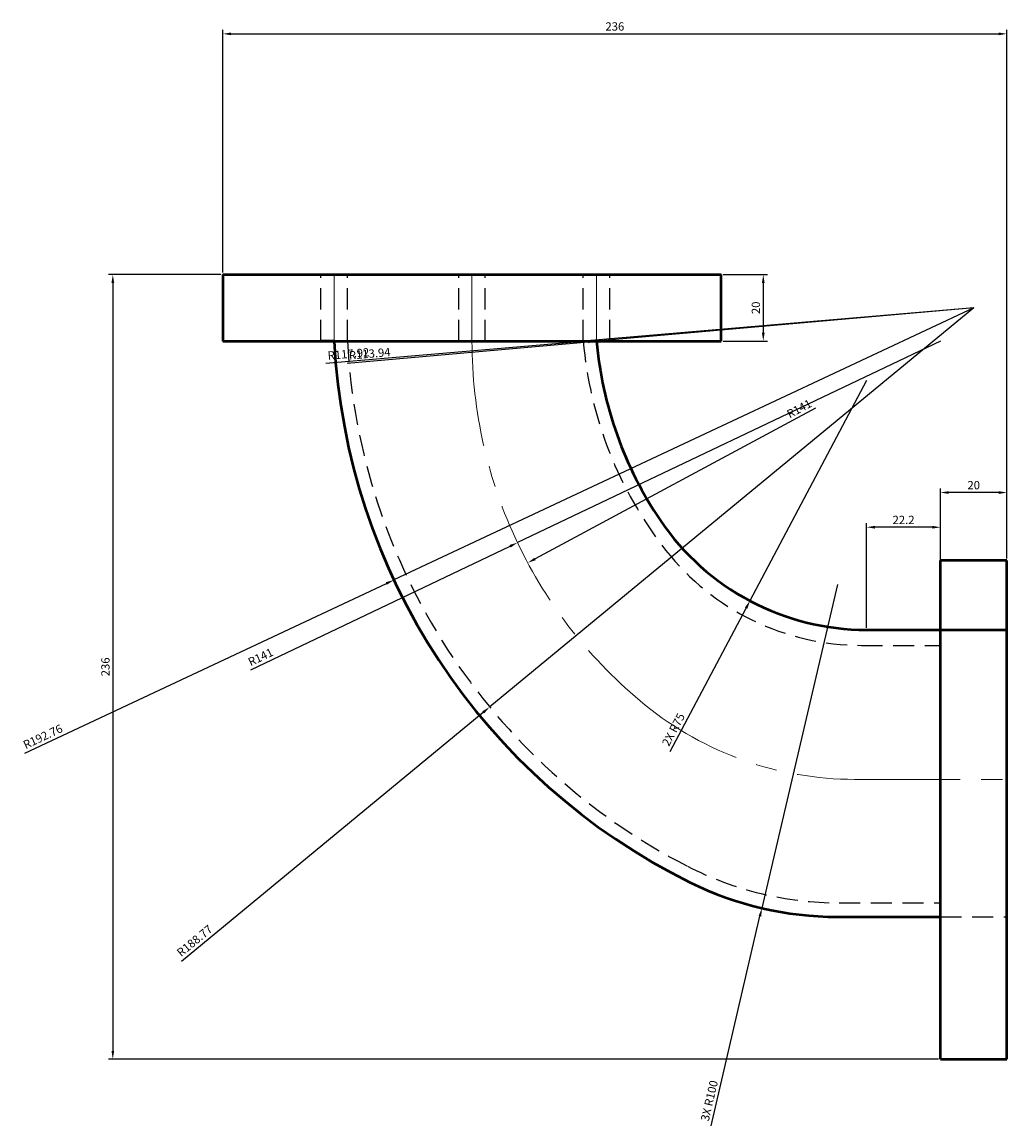
# Model space of a CAD drawing. Units: millimetres. Extents: x 1880 to 2565, y 1372 to 1704.
# Tile 1 of 2: x 1880 to 2176, y 1372 to 1704. Entities that reach past the tile are written whole.
import ezdxf

# ---------------------------------------------------------------- set-up
doc = ezdxf.new("R2010")
doc.units = ezdxf.units.MM
doc.linetypes.add('CENTER', pattern=[50.8, 31.75, -6.35, 6.35, -6.35])
doc.linetypes.add('HIDDEN', pattern=[9.525, 6.35, -3.175])
for name, color, linetype, lineweight in [('M-CNTR', 4, 'CENTER', 18), ('M-DIMS', 2, 'Continuous', 25), ('M-HIDN', 8, 'HIDDEN', 25), ('M-OUTL', 7, 'Continuous', 50)]:
    doc.layers.add(name, color=color, linetype=linetype, lineweight=lineweight)
doc.styles.get("Standard").update_dxf_attribs({"font": 'arial.ttf'})
doc.dimstyles.new('ISO-25', dxfattribs={"dimtxt": 2.5, "dimasz": 2.5, "dimexe": 1.25, "dimexo": 0.625, "dimtad": 1, "dimdec": 1, "dimdsep": 46, "dimtxsty": 'Standard', "dimcen": 2.5, "dimadec": 0, "dimazin": 0, "dimtfac": 1, "dimtdec": 1, "dimtmove": 0, "dimatfit": 3, "dimfxl": 1, "dimarcsym": 0})

# ---------------------------------------------------------------- blocks, each defined once
blk = doc.blocks.new('*D9')
at = {"layer": 'Defpoints', "color": 0, "lineweight": 100, "transparency": 16777216}
for p in [(2155.98, 1607.95), (2031.76, 1541.23)]:
    blk.add_point(p, dxfattribs=at)
at = {"layer": 'M-DIMS', "color": 0, "lineweight": -2, "transparency": 16777216}
blk.add_line((2118.32, 1587.72), (2033.97, 1542.42), dxfattribs=at)
at = {"layer": 'M-DIMS', "color": 0, "lineweight": 100, "transparency": 16777216}
blk.add_solid([(2033.77, 1542.78), (2034.16, 1542.05), (2031.76, 1541.23)], dxfattribs=at)
at = {"layer": 'M-DIMS', "color": 0, "transparency": 16777216, "insert": (2113.61, 1587.32), "char_height": 2.5, "attachment_point": 5, "rotation": 28.2384}
blk.add_mtext('R141', dxfattribs=at)
blk = doc.blocks.new('*D10')
at = {"layer": 'Defpoints', "color": 0, "lineweight": 100, "transparency": 16777216}
for p in [(2089.98, 1627.95), (2089.98, 1607.95), (2102.65, 1607.95)]:
    blk.add_point(p, dxfattribs=at)
at = {"layer": 'M-DIMS', "color": 0, "lineweight": -2, "transparency": 16777216}
for p, q in [((2090.61, 1627.95), (2103.9, 1627.95)), ((2102.65, 1625.45), (2102.65, 1610.45)), ((2090.61, 1607.95), (2103.9, 1607.95))]:
    blk.add_line(p, q, dxfattribs=at)
at = {"layer": 'M-DIMS', "color": 0, "lineweight": 100, "transparency": 16777216}
for points in [[(2102.23, 1625.45), (2103.06, 1625.45), (2102.65, 1627.95)], [(2102.23, 1610.45), (2103.06, 1610.45), (2102.65, 1607.95)]]:
    blk.add_solid(points, dxfattribs=at)
at = {"layer": 'M-DIMS', "color": 0, "transparency": 16777216, "insert": (2100.74, 1617.95), "char_height": 2.5, "attachment_point": 5, "rotation": 90}
blk.add_mtext('20', dxfattribs=at)
blk = doc.blocks.new('*D11')
at = {"layer": 'Defpoints', "color": 0, "lineweight": 100, "transparency": 16777216}
for p in [(2133.76, 1551.95), (2133.76, 1521.08), (2155.98, 1521.08)]:
    blk.add_point(p, dxfattribs=at)
at = {"layer": 'M-DIMS', "color": 0, "lineweight": -2, "transparency": 16777216}
for p, q in [((2133.76, 1521.71), (2133.76, 1553.2)), ((2153.48, 1551.95), (2136.26, 1551.95)), ((2155.98, 1521.71), (2155.98, 1553.2))]:
    blk.add_line(p, q, dxfattribs=at)
at = {"layer": 'M-DIMS', "color": 0, "lineweight": 100, "transparency": 16777216}
for points in [[(2136.26, 1552.36), (2136.26, 1551.53), (2133.76, 1551.95)], [(2153.48, 1552.36), (2153.48, 1551.53), (2155.98, 1551.95)]]:
    blk.add_solid(points, dxfattribs=at)
at = {"layer": 'M-DIMS', "color": 0, "transparency": 16777216, "insert": (2144.87, 1553.83), "char_height": 2.5, "attachment_point": 5}
blk.add_mtext('22.2', dxfattribs=at)
blk = doc.blocks.new('*D12')
at = {"layer": 'Defpoints', "color": 0, "lineweight": 100, "transparency": 16777216}
for p in [(2155.98, 1562.38), (2155.98, 1541.95), (2175.98, 1541.95)]:
    blk.add_point(p, dxfattribs=at)
at = {"layer": 'M-DIMS', "color": 0, "lineweight": -2, "transparency": 16777216}
for p, q in [((2155.98, 1542.57), (2155.98, 1563.63)), ((2173.48, 1562.38), (2158.48, 1562.38)), ((2175.98, 1542.57), (2175.98, 1563.63))]:
    blk.add_line(p, q, dxfattribs=at)
at = {"layer": 'M-DIMS', "color": 0, "lineweight": 100, "transparency": 16777216}
for points in [[(2158.48, 1562.8), (2158.48, 1561.97), (2155.98, 1562.38)], [(2173.48, 1562.8), (2173.48, 1561.97), (2175.98, 1562.38)]]:
    blk.add_solid(points, dxfattribs=at)
at = {"layer": 'M-DIMS', "color": 0, "transparency": 16777216, "insert": (2165.98, 1564.29), "char_height": 2.5, "attachment_point": 5}
blk.add_mtext('20', dxfattribs=at)
blk = doc.blocks.new('FLANGE-150x20-EDGE')
for p, q in [((0, 20), (150, 20)), ((0, 20), (0, 0)), ((150, 0), (150, 20)), ((0, 0), (150, 0))]:
    blk.add_line(p, q)
blk = doc.blocks.new('*D14')
at = {"layer": 'Defpoints', "color": 0, "lineweight": 100, "transparency": 16777216}
for p in [(2175.98, 1700.35), (1939.98, 1627.95), (2175.98, 1541.95)]:
    blk.add_point(p, dxfattribs=at)
at = {"layer": 'M-DIMS', "color": 0, "lineweight": -2, "transparency": 16777216}
for p, q in [((1939.98, 1628.57), (1939.98, 1701.6)), ((1942.48, 1700.35), (2173.48, 1700.35)), ((2175.98, 1542.57), (2175.98, 1701.6))]:
    blk.add_line(p, q, dxfattribs=at)
at = {"layer": 'M-DIMS', "color": 0, "lineweight": 100, "transparency": 16777216}
for points in [[(1942.48, 1700.77), (1942.48, 1699.94), (1939.98, 1700.35)], [(2173.48, 1700.77), (2173.48, 1699.94), (2175.98, 1700.35)]]:
    blk.add_solid(points, dxfattribs=at)
at = {"layer": 'M-DIMS', "color": 0, "transparency": 16777216, "insert": (2057.98, 1702.26), "char_height": 2.5, "attachment_point": 5}
blk.add_mtext('236', dxfattribs=at)
blk = doc.blocks.new('*D15')
at = {"layer": 'Defpoints', "color": 0, "lineweight": 100, "transparency": 16777216}
for p in [(1939.98, 1627.95), (1906.88, 1391.95), (2155.98, 1391.95)]:
    blk.add_point(p, dxfattribs=at)
at = {"layer": 'M-DIMS', "color": 0, "lineweight": -2, "transparency": 16777216}
for p, q in [((1939.36, 1627.95), (1905.63, 1627.95)), ((1906.88, 1625.45), (1906.88, 1394.45)), ((2155.36, 1391.95), (1905.63, 1391.95))]:
    blk.add_line(p, q, dxfattribs=at)
at = {"layer": 'M-DIMS', "color": 0, "lineweight": 100, "transparency": 16777216}
for points in [[(1906.47, 1625.45), (1907.3, 1625.45), (1906.88, 1627.95)], [(1906.47, 1394.45), (1907.3, 1394.45), (1906.88, 1391.95)]]:
    blk.add_solid(points, dxfattribs=at)
at = {"layer": 'M-DIMS', "color": 0, "transparency": 16777216, "insert": (1904.98, 1509.95), "char_height": 2.5, "attachment_point": 5, "rotation": 90}
blk.add_mtext('236', dxfattribs=at)
blk = doc.blocks.new('*D17')
at = {"layer": 'Defpoints', "color": 0, "lineweight": 100, "transparency": 16777216}
for p in [(2165.98, 1617.95), (1991.47, 1536.08)]:
    blk.add_point(p, dxfattribs=at)
at = {"layer": 'M-DIMS', "color": 0, "lineweight": -2, "transparency": 16777216}
for p, q in [((2165.98, 1617.95), (1991.47, 1536.08)), ((1880.42, 1483.98), (1989.21, 1535.02))]:
    blk.add_line(p, q, dxfattribs=at)
at = {"layer": 'M-DIMS', "color": 0, "lineweight": 100, "transparency": 16777216}
blk.add_solid([(1989.03, 1535.4), (1989.38, 1534.64), (1991.47, 1536.08)], dxfattribs=at)
at = {"layer": 'M-DIMS', "color": 0, "transparency": 16777216, "insert": (1885.96, 1488.68), "char_height": 2.5, "attachment_point": 5, "rotation": 25.1319}
blk.add_mtext('R192.76', dxfattribs=at)
blk = doc.blocks.new('*D18')
at = {"layer": 'Defpoints', "color": 0, "lineweight": 100, "transparency": 16777216}
for p in [(2165.98, 1617.95), (2020.32, 1497.89)]:
    blk.add_point(p, dxfattribs=at)
at = {"layer": 'M-DIMS', "color": 0, "lineweight": -2, "transparency": 16777216}
for p, q in [((2165.98, 1617.95), (2020.32, 1497.89)), ((1927.51, 1421.39), (2018.39, 1496.3))]:
    blk.add_line(p, q, dxfattribs=at)
at = {"layer": 'M-DIMS', "color": 0, "lineweight": 100, "transparency": 16777216}
blk.add_solid([(2018.12, 1496.62), (2018.65, 1495.97), (2020.32, 1497.89)], dxfattribs=at)
at = {"layer": 'M-DIMS', "color": 0, "transparency": 16777216, "insert": (1931.71, 1427.32), "char_height": 2.5, "attachment_point": 5, "rotation": 39.4963}
blk.add_mtext('R188.77', dxfattribs=at)
blk = doc.blocks.new('*D19')
at = {"layer": 'Defpoints', "color": 0, "lineweight": 100, "transparency": 16777216}
for p in [(2155.98, 1607.95), (2028.69, 1547.31)]:
    blk.add_point(p, dxfattribs=at)
at = {"layer": 'M-DIMS', "color": 0, "lineweight": -2, "transparency": 16777216}
for p, q in [((2155.98, 1607.95), (2028.69, 1547.31)), ((1948.39, 1509.06), (2026.43, 1546.23))]:
    blk.add_line(p, q, dxfattribs=at)
at = {"layer": 'M-DIMS', "color": 0, "lineweight": 100, "transparency": 16777216}
blk.add_solid([(2026.25, 1546.61), (2026.61, 1545.86), (2028.69, 1547.31)], dxfattribs=at)
at = {"layer": 'M-DIMS', "color": 0, "transparency": 16777216, "insert": (1951.5, 1512.62), "char_height": 2.5, "attachment_point": 5, "rotation": 25.471}
blk.add_mtext('R141', dxfattribs=at)
blk = doc.blocks.new('*D20')
at = {"layer": 'Defpoints', "color": 0, "lineweight": 100, "transparency": 16777216}
for p in [(2165.98, 1617.95), (2052.48, 1607.94)]:
    blk.add_point(p, dxfattribs=at)
at = {"layer": 'M-DIMS', "color": 0, "lineweight": -2, "transparency": 16777216}
for p, q in [((2165.98, 1617.95), (2052.48, 1607.94)), ((1977.4, 1601.32), (2049.99, 1607.72))]:
    blk.add_line(p, q, dxfattribs=at)
at = {"layer": 'M-DIMS', "color": 0, "lineweight": 100, "transparency": 16777216}
blk.add_solid([(2049.96, 1608.14), (2050.03, 1607.31), (2052.48, 1607.94)], dxfattribs=at)
at = {"layer": 'M-DIMS', "color": 0, "transparency": 16777216, "insert": (1984.22, 1603.83), "char_height": 2.5, "attachment_point": 5, "rotation": 5.0379}
blk.add_mtext('R113.94', dxfattribs=at)
blk = doc.blocks.new('*D21')
at = {"layer": 'Defpoints', "color": 0, "lineweight": 100, "transparency": 16777216}
for p in [(2165.98, 1617.95), (2048.49, 1607.9)]:
    blk.add_point(p, dxfattribs=at)
at = {"layer": 'M-DIMS', "color": 0, "lineweight": -2, "transparency": 16777216}
for p, q in [((2165.98, 1617.95), (2048.49, 1607.9)), ((1971.02, 1601.28), (2046, 1607.69))]:
    blk.add_line(p, q, dxfattribs=at)
at = {"layer": 'M-DIMS', "color": 0, "lineweight": 100, "transparency": 16777216}
blk.add_solid([(2045.96, 1608.1), (2046.03, 1607.27), (2048.49, 1607.9)], dxfattribs=at)
at = {"layer": 'M-DIMS', "color": 0, "transparency": 16777216, "insert": (1977.83, 1603.77), "char_height": 2.5, "attachment_point": 5, "rotation": 4.8858}
blk.add_mtext('R117.92', dxfattribs=at)
blk = doc.blocks.new('*D22')
at = {"layer": 'Defpoints', "color": 0, "lineweight": 100, "transparency": 16777216}
for p in [(2124.94, 1534.76), (2102.22, 1437.38)]:
    blk.add_point(p, dxfattribs=at)
at = {"layer": 'M-DIMS', "color": 0, "lineweight": -2, "transparency": 16777216}
for p, q in [((2124.94, 1534.76), (2102.22, 1437.38)), ((2086.93, 1371.87), (2101.65, 1434.94))]:
    blk.add_line(p, q, dxfattribs=at)
at = {"layer": 'M-DIMS', "color": 0, "lineweight": 100, "transparency": 16777216}
blk.add_solid([(2101.24, 1435.04), (2102.05, 1434.85), (2102.22, 1437.38)], dxfattribs=at)
at = {"layer": 'M-DIMS', "color": 0, "transparency": 16777216, "insert": (2086.73, 1379.38), "char_height": 2.5, "attachment_point": 5, "rotation": 76.8678}
blk.add_mtext('3X R100', dxfattribs=at)
blk = doc.blocks.new('*D23')
at = {"layer": 'Defpoints', "color": 0, "lineweight": 100, "transparency": 16777216}
for p in [(2133.76, 1596.08), (2098.64, 1529.82)]:
    blk.add_point(p, dxfattribs=at)
at = {"layer": 'M-DIMS', "color": 0, "lineweight": -2, "transparency": 16777216}
for p, q in [((2133.76, 1596.08), (2098.64, 1529.82)), ((2074.6, 1484.46), (2097.47, 1527.61))]:
    blk.add_line(p, q, dxfattribs=at)
at = {"layer": 'M-DIMS', "color": 0, "lineweight": 100, "transparency": 16777216}
blk.add_solid([(2097.1, 1527.8), (2097.84, 1527.41), (2098.64, 1529.82)], dxfattribs=at)
at = {"layer": 'M-DIMS', "color": 0, "transparency": 16777216, "insert": (2075.89, 1490.94), "char_height": 2.5, "attachment_point": 5, "rotation": 62.0774}
blk.add_mtext('2X R75', dxfattribs=at)

msp = doc.modelspace()

# ---------------------------------------------------------------- linework, layer by layer
at = {"layer": 'M-CNTR'}
for p, q in [((1973.482, 1607.946), (1973.482, 1627.946)), ((2014.982, 1607.946), (2014.982, 1627.946)), ((2052.482, 1607.946), (2052.482, 1627.946)), ((2130.148, 1476.109), (2175.982, 1476.109))]:
    msp.add_line(p, q, dxfattribs=at)
for centre, radius, start, end in [((2155.982, 1607.946), 141, 180, 230.94238), ((2130.148, 1576.109), 100, 230.94238, 270)]:
    msp.add_arc(centre, radius, start, end, dxfattribs=at)
at = {"layer": 'M-HIDN'}
for p, q in [((1969.482, 1607.946), (1969.482, 1627.946)), ((1977.482, 1607.946), (1977.482, 1627.946)), ((2010.982, 1607.946), (2010.982, 1627.946)), ((2018.982, 1607.946), (2018.982, 1627.946)), ((2048.482, 1607.946), (2048.482, 1627.946)), ((2056.482, 1607.946), (2056.482, 1627.946)), ((2132.23, 1516.426), (2155.982, 1516.426)), ((2125.46, 1438.97), (2155.982, 1438.97)), ((2155.982, 1434.762), (2175.982, 1434.762))]:
    msp.add_line(p, q, dxfattribs=at)
for centre, radius, start, end in [((2165.982, 1617.946), 188.765, 183.03672, 242.83738), ((2165.982, 1617.946), 117.925, 184.86451, 218.15699), ((2132.23, 1591.426), 75, 218.15699, 270), ((2125.46, 1538.97), 100, 242.83738, 270)]:
    msp.add_arc(centre, radius, start, end, dxfattribs=at)
at = {"layer": 'M-OUTL'}
for p, q in [((1973.482, 1607.946), (1969.482, 1607.946)), ((2133.759, 1521.084), (2175.982, 1521.084)), ((2124.936, 1434.762), (2155.982, 1434.762))]:
    msp.add_line(p, q, dxfattribs=at)
for centre, radius, start, end in [((2165.982, 1617.946), 192.76, 182.97373, 243.73621), ((2165.982, 1617.946), 113.94, 185.03508, 214.15495), ((2133.759, 1596.084), 75, 214.15495, 270), ((2124.936, 1534.762), 100, 243.73621, 270)]:
    msp.add_arc(centre, radius, start, end, dxfattribs=at)

# ---------------------------------------------------------------- block references
msp.add_blockref('FLANGE-150x20-EDGE', (1939.982, 1607.946), dxfattribs=at)
at = {"layer": 'M-OUTL', "rotation": 90.00000000000021}
msp.add_blockref('FLANGE-150x20-EDGE', (2175.982, 1391.945), dxfattribs=at)

# ---------------------------------------------------------------- dimensions: what is measured, and where the dimension line sits
at = {"layer": 'M-DIMS'}
for base, p1, p2, override, picture, middle in [((2175.982, 1700.353), (1939.982, 1627.946), (2175.982, 1541.946), {"dimdec": 0, "dimlfac": 1, "dimrnd": 0, "dimzin": 0, "dimdsep": 46, "dimlunit": 2}, '*D14', (2057.982, 1702.255)), ((2155.982, 1562.384), (2175.982, 1541.946), (2155.982, 1541.946), {"dimclrd": 0, "dimclre": 0, "dimclrt": 0}, '*D12', (2165.982, 1564.286)), ((2133.759, 1551.948), (2155.982, 1521.084), (2133.759, 1521.084), {"dimclrd": 0, "dimclre": 0, "dimclrt": 0}, '*D11', (2144.871, 1553.828))]:
    dim = msp.add_linear_dim(base=base, p1=p1, p2=p2, dimstyle='ISO-25', override=override, dxfattribs=at)
    dim.commit()
    dim.dimension.update_dxf_attribs({"geometry": picture, "text_midpoint": middle})
for base, p1, p2, override, picture, middle in [((1906.882, 1391.946), (1939.982, 1627.946), (2155.982, 1391.946), {"dimdec": 0, "dimlfac": 1, "dimrnd": 0, "dimzin": 0, "dimdsep": 46, "dimlunit": 2}, '*D15', (1904.98, 1509.946)), ((2102.646, 1607.946), (2089.982, 1627.946), (2089.982, 1607.946), {"dimclrd": 0, "dimclre": 0, "dimclrt": 0}, '*D10', (2100.745, 1617.946))]:
    dim = msp.add_linear_dim(base=base, p1=p1, p2=p2, angle=90, dimstyle='ISO-25', override=override, dxfattribs=at)
    dim.commit()
    dim.dimension.update_dxf_attribs({"geometry": picture, "text_midpoint": middle})
for center, mpoint, override, picture, middle in [((2165.982, 1617.946), (1991.471, 1536.08), {"dimdec": 2, "dimlfac": 1, "dimrnd": 0, "dimzin": 0, "dimdsep": 46, "dimlunit": 2}, '*D17', (1886.764, 1486.961)), ((2165.98234, 1617.94564), (2020.31876, 1497.88577), {"dimdec": 2, "dimlfac": 1, "dimrnd": 0, "dimzin": 0, "dimdsep": 46, "dimlunit": 2}, '*D18', (1932.92061, 1425.84985)), ((2165.982, 1617.946), (2048.486, 1607.902), {"dimdec": 2, "dimlfac": 1, "dimrnd": 0, "dimzin": 0, "dimdsep": 46, "dimlunit": 2}, '*D21', (1977.988, 1601.876)), ((2165.982, 1617.946), (2052.483, 1607.94), {"dimdec": 2, "dimlfac": 1, "dimrnd": 0, "dimzin": 0, "dimdsep": 46, "dimlunit": 2}, '*D20', (1984.383, 1601.937)), ((2155.982, 1607.946), (2028.687, 1547.308), {"dimdec": 0, "dimlfac": 1, "dimrnd": 0, "dimzin": 0, "dimdsep": 46, "dimlunit": 2}, '*D19', (1952.31, 1510.925)), ((2155.982, 1607.946), (2031.763, 1541.233), {"dimclrd": 0, "dimclre": 0, "dimclrt": 0}, '*D9', (2114.498, 1585.666))]:
    dim = msp.add_radius_dim(center=center, mpoint=mpoint, dimstyle='ISO-25', override=override, dxfattribs=at)
    dim.commit()
    dim.dimension.update_dxf_attribs({"geometry": picture, "text_midpoint": middle, "dimtype": 164})
for center, mpoint, text, picture, middle in [((2133.759, 1596.084), (2098.638, 1529.815), '2X <>', '*D23', (2077.566, 1490.054)), ((2124.936, 1534.762), (2102.216, 1437.377), '3X <>', '*D22', (2088.584, 1378.946))]:
    dim = msp.add_radius_dim(center=center, mpoint=mpoint, text=text, dimstyle='ISO-25', override={"dimdec": 0, "dimlfac": 1, "dimrnd": 0, "dimzin": 0, "dimdsep": 46, "dimlunit": 2}, dxfattribs=at)
    dim.commit()
    dim.dimension.update_dxf_attribs({"geometry": picture, "text_midpoint": middle, "dimtype": 164})

doc.saveas('drawing.dxf')
